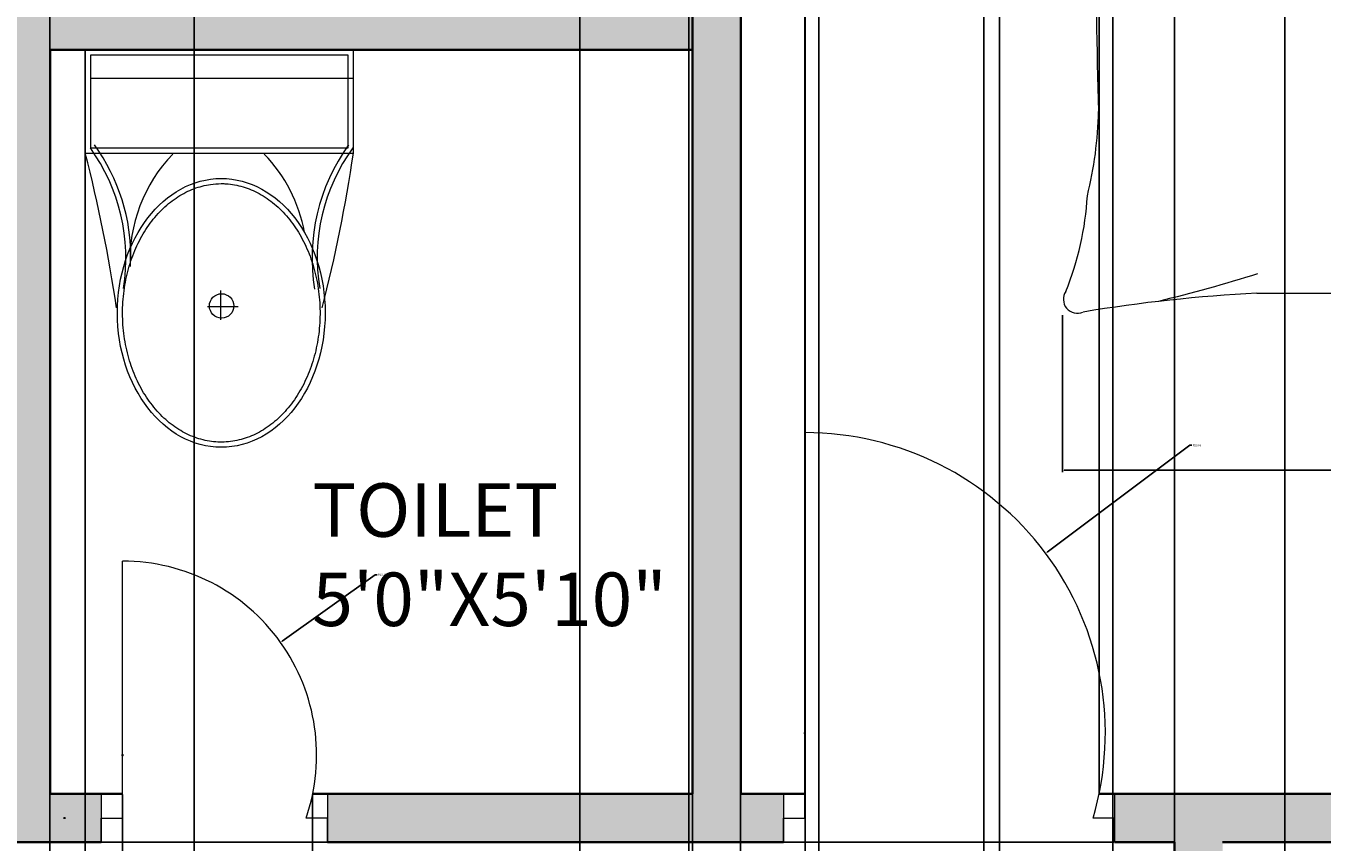
# Model space of a CAD drawing. Units: inches. Extents: x 2606 to 3027, y 1906 to 2463.
# Tile 7 of 10: x 2785 to 2906, y 2253 to 2329. Entities that reach past the tile are written whole.
import ezdxf

# ---------------------------------------------------------------- set-up
doc = ezdxf.new("R2010")
doc.units = ezdxf.units.IN
for name, color, linetype, lineweight in [('A-ANNO-DIMS', 2, 'Continuous', 18), ('A-AREA-IDEN', 7, 'Continuous', 18), ('A-DOOR', 3, 'Continuous', 18), ('A-FLOR-FIXT', 9, 'Continuous', 18), ('A-FURN', 8, 'Continuous', 13), ('A-WALL', 7, 'Continuous', 35)]:
    doc.layers.add(name, color=color, linetype=linetype, lineweight=lineweight)
doc.layers.add('A-WALL-PATT', color=251, linetype='Continuous', lineweight=13, true_color=0x636466)
doc.styles.get("Standard").update_dxf_attribs({"font": 'arial.ttf'})
doc.dimstyles.get("Standard").update_dxf_attribs({"dimtxt": 0.18, "dimasz": 0.18, "dimexe": 0.18, "dimexo": 0.0625, "dimgap": 0.09, "dimtad": 0, "dimtih": 1, "dimtoh": 1, "dimdec": 4, "dimzin": 0, "dimdsep": 46, "dimtxsty": 'Standard', "dimcen": 0.09, "dimadec": 0, "dimazin": 0, "dimtfac": 1, "dimtdec": 4, "dimtofl": 0, "dimtmove": 0, "dimatfit": 3, "dimfxl": 1, "dimtolj": 1, "dimtzin": 0, "dimarcsym": 0})

# ---------------------------------------------------------------- blocks, each defined once
blk = doc.blocks.new('A$C31115884')
for p, q in [((257.5, 466.4), (257.5, 523.2)), ((283.1, 497.7), (223.4, 497.7)), ((0, 200), (0, 0)), ((520, 200), (0, 200)), ((10, 190), (10, 10)), ((510, 190), (10, 190)), ((510, 10), (510, 190)), ((520, 0), (520, 200)), ((510, 54.5), (0, 54.5)), ((10, 10), (510, 10)), ((0, 0), (520, 0))]:
    blk.add_line(p, q)
blk.add_circle((255.6, 496.4), 23.6)
for centre, radius, start, end in [((2777.7, -204.6), 2807, 165.4549, 171.7133), ((3237, 905), 2807, 188.2867, 194.5451), ((-294.5, 403.3), 364.7, 324.2091, 9.3499), ((-294.5, 403.3), 374.7, 324.2091, 9.3499), ((805.8, 403.3), 364.7, 170.6501, 215.7909), ((139.5, 406.2), 293.5, 315.8436, 2.6563), ((805.8, 403.3), 374.7, 179.2036, 215.7909), ((383.6, 406.2), 293.5, 190.2774, 224.1564)]:
    blk.add_arc(centre, radius, start, end)
blk.add_ellipse((256.2, 509.9), major_axis=(0, -260.7), ratio=0.772727)
blk.add_open_spline([(256.2, 259.2), (263.1, 259.2), (270, 259.7), (287.8, 262.3), (298.7, 265.1), (319.9, 273.1), (330.2, 278.4), (350.1, 291.1), (359.7, 298.7), (377.7, 315.9), (386.2, 325.5), (401.7, 346.6), (408.8, 358.1), (421.3, 382.5), (426.8, 395.5), (435.9, 422.4), (439.5, 436.4), (444.8, 465.1), (446.5, 479.7), (447.9, 509.2), (447.6, 524), (445, 553.3), (442.7, 567.8), (436.3, 596), (432.1, 609.7), (421.9, 636), (416, 648.6), (402.5, 672.1), (395, 683), (378.6, 703), (369.8, 712.1), (351.1, 728), (341.3, 734.8), (320.9, 746.2), (310.4, 750.7), (288.9, 757.3), (278, 759.4), (256, 761), (245, 760.6), (223.1, 757.2), (212.3, 754.3), (191.1, 746.1), (180.8, 740.7), (160.9, 727.8), (151.4, 720.1), (133.5, 702.7), (125.1, 693), (109.6, 671.7), (102.6, 660.2), (90.2, 635.7), (84.9, 622.7), (76, 595.6), (72.4, 581.6), (67.2, 552.9), (65.6, 538.2), (64.4, 508.8), (64.8, 494), (67.5, 464.7), (69.9, 450.2), (76.6, 422), (80.8, 408.3), (91.1, 382.2), (97.2, 369.7), (110.8, 346.3), (118.4, 335.4), (134.8, 315.6), (143.7, 306.7), (162.4, 290.9), (172.3, 284.2), (192.8, 273), (203.3, 268.6), (224.8, 262.2), (235.8, 260.2), (249.9, 259.3), (253, 259.2), (256.2, 259.2)], degree=3, knots=[0, 0, 0, 0, 0.110105, 0.110105, 0.285049, 0.285049, 0.459994, 0.459994, 0.634938, 0.634938, 0.809882, 0.809882, 0.984827, 0.984827, 1.159771, 1.159771, 1.334715, 1.334715, 1.50966, 1.50966, 1.684604, 1.684604, 1.859549, 1.859549, 2.034493, 2.034493, 2.209437, 2.209437, 2.384382, 2.384382, 2.559326, 2.559326, 2.73427, 2.73427, 2.909215, 2.909215, 3.084159, 3.084159, 3.259103, 3.259103, 3.434048, 3.434048, 3.608992, 3.608992, 3.783936, 3.783936, 3.958881, 3.958881, 4.133825, 4.133825, 4.30877, 4.30877, 4.483714, 4.483714, 4.658658, 4.658658, 4.833603, 4.833603, 5.008547, 5.008547, 5.183491, 5.183491, 5.358436, 5.358436, 5.53338, 5.53338, 5.708324, 5.708324, 5.883269, 5.883269, 6.058213, 6.058213, 6.233158, 6.233158, 6.283185, 6.283185, 6.283185, 6.283185])
blk = doc.blocks.new('BED-DOUBLE')
for p, q in [((4.17, 75.16), (4.17, 96.87)), ((4.17, 96.87), (61.46, 96.87)), ((61.46, 96.87), (61.46, 64.97)), ((4.17, 95.03), (61.46, 95.03)), ((29.42, 93.94), (31.15, 94.63)), ((31.15, 94.63), (31.84, 88.22)), ((4.67, 92.87), (9.81, 93.27)), ((9.81, 93.27), (9.93, 93.24)), ((9.93, 93.24), (14.52, 92.9)), ((17.81, 92.38), (20.24, 93.24)), ((20.24, 93.24), (23.7, 94.11)), ((23.7, 94.11), (24.09, 94.11)), ((24.09, 94.11), (29.42, 93.94)), ((33.54, 93.89), (33.25, 87.44)), ((35.31, 93.3), (33.54, 93.89)), ((40.62, 93.81), (35.31, 93.3)), ((41.01, 93.83), (40.62, 93.81)), ((44.52, 93.18), (41.01, 93.83)), ((54.8, 93.82), (50.25, 93.19)), ((60.08, 93.81), (53.6, 93.92)), ((53.6, 93.92), (54.8, 93.82)), ((60.08, 93.81), (59.62, 89.96)), ((4.67, 92.9), (5.36, 89.08)), ((14.52, 92.9), (21.1, 91.68)), ((50.25, 93.19), (43.75, 91.57)), ((47, 92.47), (44.52, 93.18)), ((59.12, 86.97), (57.7, 90.18)), ((59.62, 89.96), (60.34, 86.88)), ((5.36, 89.08), (4.84, 85.96)), ((6.06, 86.14), (7.27, 89.43)), ((31.84, 88.22), (32.54, 84.4)), ((33.25, 87.44), (32.79, 83.59)), ((4.84, 85.96), (5.54, 84.75)), ((5.36, 81.8), (6.06, 86.14)), ((60.08, 82.69), (59.12, 86.97)), ((60.34, 86.88), (59.72, 85.62)), ((32.54, 84.4), (32.54, 82.84)), ((32.79, 83.59), (32.89, 82.03)), ((32.54, 82.84), (31.84, 80.59)), ((59.85, 80.77), (60.08, 82.69)), ((5.71, 79.9), (5.36, 81.8)), ((32.89, 82.03), (33.72, 79.83)), ((5.02, 76.08), (5.71, 79.9)), ((31.84, 80.59), (31.84, 77.38)), ((60.78, 77), (59.85, 80.77)), ((28.9, 77.38), (25.13, 78.68)), ((33.72, 79.83), (33.92, 76.62)), ((7.65, 78.14), (12.48, 77.34)), ((20.89, 76.82), (23.24, 77.49)), ((23.24, 77.49), (29.39, 77)), ((36.87, 76.8), (40.55, 78.34)), ((39.04, 78.14), (43.87, 77.34)), ((52.28, 76.82), (54.63, 77.49)), ((54.63, 77.49), (60.78, 77)), ((11.13, 76.95), (5.02, 76.08)), ((12.48, 77.34), (11.13, 76.95)), ((12.48, 77.34), (20.89, 76.82)), ((31.84, 77.38), (28.9, 77.38)), ((33.92, 76.62), (36.87, 76.8)), ((43.87, 77.34), (52.28, 76.82)), ((36.28, 76.03), (41.3, 68.25)), ((48.73, 72.52), (38.73, 76.03)), ((55.41, 70.1), (48.73, 72.52)), ((58.94, 67.51), (55.41, 70.1)), ((41.3, 68.25), (43.34, 62.87)), ((63.38, 63.61), (58.94, 67.51)), ((53.18, 62.87), (57.82, 63.24)), ((57.82, 63.24), (61.54, 62.87)), ((61.54, 62.87), (63.38, 63.61)), ((63.48, 61.52), (63.38, 63.61, 4.64)), ((43.34, 62.87), (43.71, 60.45)), ((46.68, 61.2), (49.1, 62.31)), ((49.1, 62.31), (53.18, 62.87)), ((43.71, 60.45), (46.68, 61.2)), ((18.06, 1.87), (47.57, 1.87))]:
    blk.add_line(p, q)
for centre, radius, start, end in [((25.61, -121.38), 197.77, 86.0865, 96.7821), ((102.1, 72.78), 99.87, 178.7218, 185.604), ((21.29, -90.53), 154.68, 81.7845, 96.9006), ((-200.58, 59.5), 203.94, 358.4762, 1.0082), ((52.44, 54.83), 7.46, 78.6608, 113.7384), ((61.53, 104.85), 43.38, 259.8763, 272.5657), ((37.35, 95.1), 35.55, 280.6617, 289.8806), ((218.51, 53.34), 155.25, 176.9791, 183.8365), ((43.92, 60.38), 0.221, 160.2464, 271.1377), ((581.23, 36.19), 578.22, 178.22771, 181.71854), ((-5405.34, 15.56), 5469.02, 0.00217, 0.28689), ((-32.25, 19.53), 35.53, 346.0648, 358.9113), ((91.3, 14.55), 27.65, 177.4714, 206.4681), ((-25.97, 12.62), 28.25, 337.9751, 356.652), ((-20.65, 125.3), 127.63, 283.3832, 287.7053), ((1.3, 1.3), 1.31, 146.1736, 293.4781), ((25.69, -143.9), 145.97, 92.9958, 99.4091), ((49.34, -157.62), 159.5, 84.4998, 90.6351), ((65.23, 2.32), 1.32, 242.6588, 356.02)]:
    blk.add_arc(centre, radius, start, end)
blk = doc.blocks.new('*D10')
at = {"layer": 'A-ANNO-DIMS', "color": 0, "lineweight": -2, "transparency": 16777216}
for p, q in [((2882.1, 2302.34), (2882.1, 2287.67)), ((2948.75, 2302.34), (2948.75, 2287.67)), ((2882.28, 2287.85), (2914.9, 2287.85)), ((2948.57, 2287.85), (2915.96, 2287.85))]:
    blk.add_line(p, q, dxfattribs=at)
at = {"layer": 'A-ANNO-DIMS', "color": 0, "transparency": 16777216}
for points in [[(2882.28, 2287.88), (2882.28, 2287.82), (2882.1, 2287.85)], [(2948.57, 2287.88), (2948.57, 2287.82), (2948.75, 2287.85)]]:
    blk.add_solid(points, dxfattribs=at)
at = {"layer": 'Defpoints', "color": 0, "transparency": 16777216}
for p in [(2882.1, 2302.4), (2948.75, 2302.4), (2948.75, 2287.85)]:
    blk.add_point(p, dxfattribs=at)
at = {"layer": 'A-ANNO-DIMS', "color": 0, "transparency": 16777216, "insert": (2915.43, 2287.85), "char_height": 0.18, "attachment_point": 5}
blk.add_mtext('\\A1;67 TYP.', dxfattribs=at)
blk = doc.blocks.new('*D34')
at = {"layer": 'A-ANNO-DIMS', "color": 0, "lineweight": -2, "transparency": 16777216}
for p, q in [((2787.56, 2118.27), (2787.56, 2433.99)), ((2787.74, 2433.81), (2817.34, 2433.81)), ((2847.38, 2433.81), (2817.78, 2433.81)), ((2847.56, 2118.27), (2847.56, 2433.99))]:
    blk.add_line(p, q, dxfattribs=at)
at = {"layer": 'A-ANNO-DIMS', "color": 0, "transparency": 16777216}
for points in [[(2787.74, 2433.84), (2787.74, 2433.78), (2787.56, 2433.81)], [(2847.38, 2433.84), (2847.38, 2433.78), (2847.56, 2433.81)]]:
    blk.add_solid(points, dxfattribs=at)
at = {"layer": 'Defpoints', "color": 0, "transparency": 16777216}
for p in [(2847.56, 2433.81), (2787.56, 2118.21), (2847.56, 2118.21)]:
    blk.add_point(p, dxfattribs=at)
at = {"layer": 'A-ANNO-DIMS', "color": 0, "transparency": 16777216, "insert": (2817.56, 2433.81), "char_height": 0.18, "attachment_point": 5}
blk.add_mtext('\\A1;60', dxfattribs=at)
blk = doc.blocks.new('*D35')
at = {"layer": 'A-ANNO-DIMS', "color": 0, "lineweight": -2, "transparency": 16777216}
for p, q in [((2801.04, 1993.17), (2801.04, 2433.99)), ((2801.22, 2433.81), (2818.82, 2433.81)), ((2836.86, 2433.81), (2819.26, 2433.81)), ((2837.04, 1993.17), (2837.04, 2433.99))]:
    blk.add_line(p, q, dxfattribs=at)
at = {"layer": 'A-ANNO-DIMS', "color": 0, "transparency": 16777216}
for points in [[(2801.22, 2433.84), (2801.22, 2433.78), (2801.04, 2433.81)], [(2836.86, 2433.84), (2836.86, 2433.78), (2837.04, 2433.81)]]:
    blk.add_solid(points, dxfattribs=at)
at = {"layer": 'Defpoints', "color": 0, "transparency": 16777216}
for p in [(2837.04, 2433.81), (2801.04, 1993.11), (2837.04, 1993.11)]:
    blk.add_point(p, dxfattribs=at)
at = {"layer": 'A-ANNO-DIMS', "color": 0, "transparency": 16777216, "insert": (2819.04, 2433.81), "char_height": 0.18, "attachment_point": 5}
blk.add_mtext('\\A1;36', dxfattribs=at)
blk = doc.blocks.new('*D36')
at = {"layer": 'A-ANNO-DIMS', "color": 0, "lineweight": -2, "transparency": 16777216}
for p, q in [((2787.56, 1993.17), (2787.56, 2433.99)), ((2787.74, 2433.81), (2793.85, 2433.81)), ((2800.86, 2433.81), (2794.76, 2433.81)), ((2801.04, 1993.17), (2801.04, 2433.99))]:
    blk.add_line(p, q, dxfattribs=at)
at = {"layer": 'A-ANNO-DIMS', "color": 0, "transparency": 16777216}
for points in [[(2787.74, 2433.84), (2787.74, 2433.78), (2787.56, 2433.81)], [(2800.86, 2433.84), (2800.86, 2433.78), (2801.04, 2433.81)]]:
    blk.add_solid(points, dxfattribs=at)
at = {"layer": 'Defpoints', "color": 0, "transparency": 16777216}
for p in [(2787.56, 2433.81), (2787.56, 1993.11), (2801.04, 1993.11)]:
    blk.add_point(p, dxfattribs=at)
at = {"layer": 'A-ANNO-DIMS', "color": 0, "transparency": 16777216, "insert": (2794.3, 2433.81), "char_height": 0.18, "attachment_point": 5}
blk.add_mtext('\\A1;13.478', dxfattribs=at)
blk = doc.blocks.new('*D38')
at = {"layer": 'A-ANNO-DIMS', "color": 0, "lineweight": -2, "transparency": 16777216}
for p, q in [((2783.06, 1993.17), (2783.06, 2433.99)), ((2783.24, 2433.81), (2785.05, 2433.81)), ((2787.38, 2433.81), (2785.57, 2433.81)), ((2787.56, 1993.17), (2787.56, 2433.99))]:
    blk.add_line(p, q, dxfattribs=at)
at = {"layer": 'A-ANNO-DIMS', "color": 0, "transparency": 16777216}
for points in [[(2783.24, 2433.84), (2783.24, 2433.78), (2783.06, 2433.81)], [(2787.38, 2433.84), (2787.38, 2433.78), (2787.56, 2433.81)]]:
    blk.add_solid(points, dxfattribs=at)
at = {"layer": 'Defpoints', "color": 0, "transparency": 16777216}
for p in [(2787.56, 2433.81), (2783.06, 1993.11), (2787.56, 1993.11)]:
    blk.add_point(p, dxfattribs=at)
at = {"layer": 'A-ANNO-DIMS', "color": 0, "transparency": 16777216, "insert": (2785.31, 2433.81), "char_height": 0.18, "attachment_point": 5}
blk.add_mtext('\\A1;4.5', dxfattribs=at)
blk = doc.blocks.new('*D43')
at = {"layer": 'A-ANNO-DIMS', "color": 0, "lineweight": -2, "transparency": 16777216}
for p, q in [((2794.34, 2257.55), (2794.34, 1965.23)), ((2812.09, 2257.55), (2812.09, 1965.23)), ((2794.52, 1965.41), (2802.76, 1965.41)), ((2811.91, 1965.41), (2803.67, 1965.41))]:
    blk.add_line(p, q, dxfattribs=at)
at = {"layer": 'A-ANNO-DIMS', "color": 0, "transparency": 16777216}
for points in [[(2794.52, 1965.44), (2794.52, 1965.38), (2794.34, 1965.41)], [(2811.91, 1965.44), (2811.91, 1965.38), (2812.09, 1965.41)]]:
    blk.add_solid(points, dxfattribs=at)
at = {"layer": 'Defpoints', "color": 0, "transparency": 16777216}
for p in [(2794.34, 2257.61), (2812.09, 2257.61), (2812.09, 1965.41)]:
    blk.add_point(p, dxfattribs=at)
at = {"layer": 'A-ANNO-DIMS', "color": 0, "transparency": 16777216, "insert": (2803.22, 1965.41), "char_height": 0.18, "attachment_point": 5}
blk.add_mtext('\\A1;17.756', dxfattribs=at)
blk = doc.blocks.new('*D44')
at = {"layer": 'A-ANNO-DIMS', "color": 0, "lineweight": -2, "transparency": 16777216}
for p, q in [((2858.06, 2257.67), (2858.06, 2433.99)), ((2858.24, 2433.81), (2871.33, 2433.81)), ((2885.35, 2433.81), (2872.26, 2433.81)), ((2885.53, 2257.67), (2885.53, 2433.99))]:
    blk.add_line(p, q, dxfattribs=at)
at = {"layer": 'A-ANNO-DIMS', "color": 0, "transparency": 16777216}
for points in [[(2858.24, 2433.84), (2858.24, 2433.78), (2858.06, 2433.81)], [(2885.35, 2433.84), (2885.35, 2433.78), (2885.53, 2433.81)]]:
    blk.add_solid(points, dxfattribs=at)
at = {"layer": 'Defpoints', "color": 0, "transparency": 16777216}
for p in [(2885.53, 2433.81), (2858.06, 2257.61), (2885.53, 2257.61)]:
    blk.add_point(p, dxfattribs=at)
at = {"layer": 'A-ANNO-DIMS', "color": 0, "transparency": 16777216, "insert": (2871.79, 2433.81), "char_height": 0.18, "attachment_point": 5}
blk.add_mtext('\\A1;27.475', dxfattribs=at)
blk = doc.blocks.new('*D46')
at = {"layer": 'A-ANNO-DIMS', "color": 0, "lineweight": -2, "transparency": 16777216}
for p, q in [((2859.37, 2154.92), (2859.37, 2433.99)), ((2859.55, 2433.81), (2872.63, 2433.81)), ((2886.63, 2433.81), (2873.56, 2433.81)), ((2886.81, 2157.17), (2886.81, 2433.99))]:
    blk.add_line(p, q, dxfattribs=at)
at = {"layer": 'A-ANNO-DIMS', "color": 0, "transparency": 16777216}
for points in [[(2859.55, 2433.84), (2859.55, 2433.78), (2859.37, 2433.81)], [(2886.63, 2433.84), (2886.63, 2433.78), (2886.81, 2433.81)]]:
    blk.add_solid(points, dxfattribs=at)
at = {"layer": 'Defpoints', "color": 0, "transparency": 16777216}
for p in [(2886.81, 2433.81), (2886.81, 2157.11), (2859.37, 2154.86)]:
    blk.add_point(p, dxfattribs=at)
at = {"layer": 'A-ANNO-DIMS', "color": 0, "transparency": 16777216, "insert": (2873.09, 2433.81), "char_height": 0.18, "attachment_point": 5}
blk.add_mtext('\\A1;27.443', dxfattribs=at)
blk = doc.blocks.new('*D48')
at = {"layer": 'A-ANNO-DIMS', "color": 0, "lineweight": -2, "transparency": 16777216}
for p, q in [((2858.07, 2028.17), (2858.07, 2433.99)), ((2858.25, 2433.81), (2866.77, 2433.81)), ((2876.06, 2433.81), (2867.54, 2433.81)), ((2876.24, 2028.17), (2876.24, 2433.99))]:
    blk.add_line(p, q, dxfattribs=at)
at = {"layer": 'A-ANNO-DIMS', "color": 0, "transparency": 16777216}
for points in [[(2858.25, 2433.84), (2858.25, 2433.78), (2858.07, 2433.81)], [(2876.06, 2433.84), (2876.06, 2433.78), (2876.24, 2433.81)]]:
    blk.add_solid(points, dxfattribs=at)
at = {"layer": 'Defpoints', "color": 0, "transparency": 16777216}
for p in [(2876.24, 2433.81), (2858.07, 2028.11), (2876.24, 2028.11)]:
    blk.add_point(p, dxfattribs=at)
at = {"layer": 'A-ANNO-DIMS', "color": 0, "transparency": 16777216, "insert": (2867.16, 2433.81), "char_height": 0.18, "attachment_point": 5}
blk.add_mtext('\\A1;18.17', dxfattribs=at)
blk = doc.blocks.new('*D51')
at = {"layer": 'A-ANNO-DIMS', "color": 0, "lineweight": -2, "transparency": 16777216}
for p, q in [((2852.06, 2257.67), (2852.06, 2433.99)), ((2852.24, 2433.81), (2854.67, 2433.81)), ((2857.88, 2433.81), (2855.45, 2433.81)), ((2858.06, 2257.67), (2858.06, 2433.99))]:
    blk.add_line(p, q, dxfattribs=at)
at = {"layer": 'A-ANNO-DIMS', "color": 0, "transparency": 16777216}
for points in [[(2852.24, 2433.84), (2852.24, 2433.78), (2852.06, 2433.81)], [(2857.88, 2433.84), (2857.88, 2433.78), (2858.06, 2433.81)]]:
    blk.add_solid(points, dxfattribs=at)
at = {"layer": 'Defpoints', "color": 0, "transparency": 16777216}
for p in [(2858.06, 2433.81), (2852.06, 2257.61), (2858.06, 2257.61)]:
    blk.add_point(p, dxfattribs=at)
at = {"layer": 'A-ANNO-DIMS', "color": 0, "transparency": 16777216, "insert": (2855.06, 2433.81), "char_height": 0.18, "attachment_point": 5}
blk.add_mtext('\\A1;5.994', dxfattribs=at)
blk = doc.blocks.new('*D52')
at = {"layer": 'A-ANNO-DIMS', "color": 0, "lineweight": -2, "transparency": 16777216}
for p, q in [((2787.56, 2257.55), (2787.56, 1965.23)), ((2794.34, 2257.55), (2794.34, 1965.23)), ((2787.74, 1965.41), (2790.56, 1965.41)), ((2794.16, 1965.41), (2791.34, 1965.41))]:
    blk.add_line(p, q, dxfattribs=at)
at = {"layer": 'A-ANNO-DIMS', "color": 0, "transparency": 16777216}
for points in [[(2787.74, 1965.44), (2787.74, 1965.38), (2787.56, 1965.41)], [(2794.16, 1965.44), (2794.16, 1965.38), (2794.34, 1965.41)]]:
    blk.add_solid(points, dxfattribs=at)
at = {"layer": 'Defpoints', "color": 0, "transparency": 16777216}
for p in [(2787.56, 2257.61), (2794.34, 2257.61), (2794.34, 1965.41)]:
    blk.add_point(p, dxfattribs=at)
at = {"layer": 'A-ANNO-DIMS', "color": 0, "transparency": 16777216, "insert": (2790.95, 1965.41), "char_height": 0.18, "attachment_point": 5}
blk.add_mtext('\\A1;6.776', dxfattribs=at)
blk = doc.blocks.new('*D55')
at = {"layer": 'A-ANNO-DIMS', "color": 0, "lineweight": -2, "transparency": 16777216}
for p, q in [((2852.06, 2152.67), (2852.06, 2433.99)), ((2852.24, 2433.81), (2855.32, 2433.81)), ((2859.19, 2433.81), (2856.11, 2433.81)), ((2859.37, 2154.92), (2859.37, 2433.99))]:
    blk.add_line(p, q, dxfattribs=at)
at = {"layer": 'A-ANNO-DIMS', "color": 0, "transparency": 16777216}
for points in [[(2852.24, 2433.84), (2852.24, 2433.78), (2852.06, 2433.81)], [(2859.19, 2433.84), (2859.19, 2433.78), (2859.37, 2433.81)]]:
    blk.add_solid(points, dxfattribs=at)
at = {"layer": 'Defpoints', "color": 0, "transparency": 16777216}
for p in [(2859.37, 2433.81), (2859.37, 2154.86), (2852.06, 2152.61)]:
    blk.add_point(p, dxfattribs=at)
at = {"layer": 'A-ANNO-DIMS', "color": 0, "transparency": 16777216, "insert": (2855.72, 2433.81), "char_height": 0.18, "attachment_point": 5}
blk.add_mtext('\\A1;7.306', dxfattribs=at)
blk = doc.blocks.new('*D57')
at = {"layer": 'A-ANNO-DIMS', "color": 0, "lineweight": -2, "transparency": 16777216}
for p, q in [((2876.24, 2028.17), (2876.24, 2433.99)), ((2876.42, 2433.81), (2889.17, 2433.81)), ((2902.71, 2433.81), (2889.96, 2433.81)), ((2902.89, 2028.17), (2902.89, 2433.99))]:
    blk.add_line(p, q, dxfattribs=at)
at = {"layer": 'A-ANNO-DIMS', "color": 0, "transparency": 16777216}
for points in [[(2876.42, 2433.84), (2876.42, 2433.78), (2876.24, 2433.81)], [(2902.71, 2433.84), (2902.71, 2433.78), (2902.89, 2433.81)]]:
    blk.add_solid(points, dxfattribs=at)
at = {"layer": 'Defpoints', "color": 0, "transparency": 16777216}
for p in [(2902.89, 2433.81), (2876.24, 2028.11), (2902.89, 2028.11)]:
    blk.add_point(p, dxfattribs=at)
at = {"layer": 'A-ANNO-DIMS', "color": 0, "transparency": 16777216, "insert": (2889.57, 2433.81), "char_height": 0.18, "attachment_point": 5}
blk.add_mtext('\\A1;26.65', dxfattribs=at)
blk = doc.blocks.new('*D70')
at = {"layer": 'A-ANNO-DIMS', "color": 0, "lineweight": -2, "transparency": 16777216}
for p, q in [((2847.23, 2221.7), (2847.23, 2433.99)), ((2847.41, 2433.81), (2860.54, 2433.81)), ((2874.6, 2433.81), (2861.47, 2433.81)), ((2874.78, 2221.7), (2874.78, 2433.99))]:
    blk.add_line(p, q, dxfattribs=at)
at = {"layer": 'A-ANNO-DIMS', "color": 0, "transparency": 16777216}
for points in [[(2847.41, 2433.84), (2847.41, 2433.78), (2847.23, 2433.81)], [(2874.6, 2433.84), (2874.6, 2433.78), (2874.78, 2433.81)]]:
    blk.add_solid(points, dxfattribs=at)
at = {"layer": 'Defpoints', "color": 0, "transparency": 16777216}
for p in [(2874.78, 2433.81), (2847.23, 2221.64), (2874.78, 2221.64)]:
    blk.add_point(p, dxfattribs=at)
at = {"layer": 'A-ANNO-DIMS', "color": 0, "transparency": 16777216, "insert": (2861, 2433.81), "char_height": 0.18, "attachment_point": 5}
blk.add_mtext('\\A1;27.555', dxfattribs=at)
blk = doc.blocks.new('*D72')
at = {"layer": 'A-ANNO-DIMS', "color": 0, "lineweight": -2, "transparency": 16777216}
for p, q in [((2874.78, 2221.7), (2874.78, 2433.99)), ((2874.96, 2433.81), (2883.22, 2433.81)), ((2892.38, 2433.81), (2884.13, 2433.81)), ((2892.56, 2215.2), (2892.56, 2433.99))]:
    blk.add_line(p, q, dxfattribs=at)
at = {"layer": 'A-ANNO-DIMS', "color": 0, "transparency": 16777216}
for points in [[(2874.96, 2433.84), (2874.96, 2433.78), (2874.78, 2433.81)], [(2892.38, 2433.84), (2892.38, 2433.78), (2892.56, 2433.81)]]:
    blk.add_solid(points, dxfattribs=at)
at = {"layer": 'Defpoints', "color": 0, "transparency": 16777216}
for p in [(2892.56, 2433.81), (2874.78, 2221.64), (2892.56, 2215.13)]:
    blk.add_point(p, dxfattribs=at)
at = {"layer": 'A-ANNO-DIMS', "color": 0, "transparency": 16777216, "insert": (2883.67, 2433.81), "char_height": 0.18, "attachment_point": 5}
blk.add_mtext('\\A1;17.783', dxfattribs=at)
blk = doc.blocks.new('*D73')
at = {"layer": 'A-ANNO-DIMS', "color": 0, "lineweight": -2, "transparency": 16777216}
for p, q in [((2886.91, 2253.11), (2634.68, 2253.11)), ((2634.86, 2252.93), (2634.86, 2237.56)), ((2634.86, 2221.82), (2634.86, 2237.19)), ((2847.16, 2221.64), (2634.68, 2221.64))]:
    blk.add_line(p, q, dxfattribs=at)
at = {"layer": 'A-ANNO-DIMS', "color": 0, "transparency": 16777216}
for points in [[(2634.83, 2252.93), (2634.89, 2252.93), (2634.86, 2253.11)], [(2634.83, 2221.82), (2634.89, 2221.82), (2634.86, 2221.64)]]:
    blk.add_solid(points, dxfattribs=at)
at = {"layer": 'Defpoints', "color": 0, "transparency": 16777216}
for p in [(2634.86, 2253.11), (2886.97, 2253.11), (2847.23, 2221.64)]:
    blk.add_point(p, dxfattribs=at)
at = {"layer": 'A-ANNO-DIMS', "color": 0, "transparency": 16777216, "insert": (2634.86, 2237.37), "char_height": 0.18, "attachment_point": 5}
blk.add_mtext('\\A1;31.47', dxfattribs=at)
blk = doc.blocks.new('*D83')
at = {"layer": 'A-ANNO-DIMS', "color": 0, "lineweight": -2, "transparency": 16777216}
for p, q in [((2787.56, 2327.05), (2787.56, 1965.23)), ((2790.85, 2327.05), (2790.85, 1965.23)), ((2787.74, 1965.41), (2788.88, 1965.41)), ((2790.67, 1965.41), (2789.53, 1965.41))]:
    blk.add_line(p, q, dxfattribs=at)
at = {"layer": 'A-ANNO-DIMS', "color": 0, "transparency": 16777216}
for points in [[(2787.74, 1965.44), (2787.74, 1965.38), (2787.56, 1965.41)], [(2790.67, 1965.44), (2790.67, 1965.38), (2790.85, 1965.41)]]:
    blk.add_solid(points, dxfattribs=at)
at = {"layer": 'Defpoints', "color": 0, "transparency": 16777216}
for p in [(2787.56, 2327.11), (2790.85, 2327.11), (2790.85, 1965.41)]:
    blk.add_point(p, dxfattribs=at)
at = {"layer": 'A-ANNO-DIMS', "color": 0, "transparency": 16777216, "insert": (2789.21, 1965.41), "char_height": 0.18, "attachment_point": 5}
blk.add_mtext('\\A1;3.29', dxfattribs=at)
blk = doc.blocks.new('*D84')
at = {"layer": 'A-ANNO-DIMS', "color": 0, "lineweight": -2, "transparency": 16777216}
for p, q in [((2739.27, 2290.79), (2739.45, 2290.79)), ((2739.45, 2290.79), (2757.85, 2277.61)), ((2788.82, 2255.36), (2789, 2255.36)), ((2788.91, 2255.27), (2788.91, 2255.45))]:
    blk.add_line(p, q, dxfattribs=at)
at = {"layer": 'A-ANNO-DIMS', "color": 0, "transparency": 16777216}
blk.add_solid([(2757.87, 2277.63), (2757.84, 2277.58), (2758, 2277.5)], dxfattribs=at)
at = {"layer": 'Defpoints', "color": 0, "transparency": 16777216}
for p in [(2758, 2277.5), (2788.91, 2255.36)]:
    blk.add_point(p, dxfattribs=at)
at = {"layer": 'A-ANNO-DIMS', "color": 0, "transparency": 16777216, "insert": (2738.79, 2290.79), "char_height": 0.18, "attachment_point": 5}
blk.add_mtext('\\A1;R38.02', dxfattribs=at)
blk = doc.blocks.new('*D85')
at = {"layer": 'A-ANNO-DIMS', "color": 0, "lineweight": -2, "transparency": 16777216}
for p, q in [((2894.01, 2290.18), (2880.67, 2280.21)), ((2894.19, 2290.18), (2894.01, 2290.18)), ((2857.97, 2263.3), (2858.15, 2263.3)), ((2858.06, 2263.21), (2858.06, 2263.39))]:
    blk.add_line(p, q, dxfattribs=at)
at = {"layer": 'A-ANNO-DIMS', "color": 0, "transparency": 16777216}
blk.add_solid([(2880.66, 2280.23), (2880.69, 2280.18), (2880.53, 2280.1)], dxfattribs=at)
at = {"layer": 'Defpoints', "color": 0, "transparency": 16777216}
for p in [(2880.53, 2280.1), (2858.06, 2263.3)]:
    blk.add_point(p, dxfattribs=at)
at = {"layer": 'A-ANNO-DIMS', "color": 0, "transparency": 16777216, "insert": (2894.67, 2290.18), "char_height": 0.18, "attachment_point": 5}
blk.add_mtext('\\A1;R28.06', dxfattribs=at)
blk = doc.blocks.new('*D91')
at = {"layer": 'A-ANNO-DIMS', "color": 0, "lineweight": -2, "transparency": 16777216}
for p, q in [((2817.93, 2278.09), (2809.23, 2271.88)), ((2818.11, 2278.09), (2817.93, 2278.09)), ((2794.25, 2261.24), (2794.43, 2261.24)), ((2794.34, 2261.15), (2794.34, 2261.33))]:
    blk.add_line(p, q, dxfattribs=at)
at = {"layer": 'A-ANNO-DIMS', "color": 0, "transparency": 16777216}
blk.add_solid([(2809.21, 2271.9), (2809.25, 2271.85), (2809.09, 2271.77)], dxfattribs=at)
at = {"layer": 'Defpoints', "color": 0, "transparency": 16777216}
for p in [(2809.09, 2271.77), (2794.34, 2261.24)]:
    blk.add_point(p, dxfattribs=at)
at = {"layer": 'A-ANNO-DIMS', "color": 0, "transparency": 16777216, "insert": (2818.66, 2278.09), "char_height": 0.18, "attachment_point": 5}
blk.add_mtext('\\A1;R18.123', dxfattribs=at)

msp = doc.modelspace()

# ---------------------------------------------------------------- hatches: boundary and pattern name
at = {"layer": 'A-WALL-PATT'}
h = msp.add_hatch(color=256, dxfattribs=at)
h.dxf.hatch_style = 1
h.paths.add_polyline_path([(2667.063, 2401.6097), (2691.9697, 2401.6097), (2691.9697, 2406.1097), (2691.9697, 2410.6097), (2658.063, 2410.6097), (2658.063, 2238.7051), (2667.063, 2238.7051)])
h.paths.add_polyline_path([(2804.9965, 2406.1097), (2804.9965, 2410.6097), (2751.9697, 2410.6097), (2751.9697, 2401.6097), (2783.063, 2401.6097), (2783.063, 2257.6097), (2778.6739, 2257.6097), (2778.6739, 2253.1097), (2792.3386, 2253.1097), (2792.3386, 2255.3597), (2792.3386, 2257.6097), (2787.563, 2257.6097), (2787.563, 2327.1097), (2847.563, 2327.1097), (2847.563, 2331.6097), (2787.563, 2331.6097), (2787.563, 2401.6097), (2804.9965, 2401.6097)])
h.paths.add_polyline_path([(2889.6183, 2406.1097), (2889.6183, 2410.6097), (2828.9965, 2410.6097), (2828.9965, 2401.6097), (2831.8174, 2401.6097), (2847.563, 2401.6097), (2847.563, 2357.8311), (2849.813, 2357.8311), (2852.063, 2357.8311), (2852.063, 2401.6097), (2889.6183, 2401.6097)])
h.paths.add_polyline_path([(2977.063, 2410.6097), (2949.6183, 2410.6097), (2949.6183, 2401.6097), (2968.063, 2401.6097), (2968.063, 2157.1097), (2897.063, 2157.1097), (2897.063, 2174.1966), (2892.563, 2174.1966), (2892.563, 2157.1097), (2886.8122, 2157.1097), (2886.8122, 2152.6097), (2968.063, 2152.6097), (2968.063, 2032.6097), (2950.8911, 2032.6097), (2950.8911, 2028.1097), (2968.063, 2028.1097), (2968.063, 1993.1097), (2852.063, 1993.1097), (2852.063, 2028.1097), (2856.0743, 2028.1097), (2856.0743, 2030.3597), (2856.0743, 2032.6097), (2852.063, 2032.6097), (2852.063, 2152.6097), (2857.369, 2152.6097), (2857.369, 2154.8597), (2857.369, 2157.1097), (2847.563, 2157.1097), (2847.563, 2152.6097), (2847.563, 1993.1097), (2837.0415, 1993.1097), (2837.0415, 1988.6097), (2977.063, 1988.6097)])
h.paths.add_polyline_path([(2968.063, 2257.6097), (2886.9679, 2257.6097), (2886.9679, 2253.1097), (2892.563, 2253.1097), (2892.563, 2215.1332), (2897.063, 2215.1332), (2897.063, 2253.1097), (2968.063, 2253.1097)], flags=17)
h.paths.add_polyline_path([(2856.057, 2255.3597), (2856.057, 2257.6097), (2852.063, 2257.6097), (2852.063, 2336.7476), (2849.813, 2336.7476), (2847.563, 2336.7476), (2847.563, 2331.6097), (2847.563, 2327.1097), (2847.563, 2257.6097), (2813.482, 2257.6097), (2813.482, 2253.1097), (2856.057, 2253.1097)])
h.paths.add_polyline_path([(2748.8874, 2255.3597), (2748.8874, 2257.6097), (2667.063, 2257.6097), (2667.063, 2253.1097), (2748.8874, 2253.1097)])
h.paths.add_polyline_path([(2667.063, 2152.6097), (2744.8238, 2152.6097), (2744.8238, 2154.8597), (2744.8238, 2157.1097), (2667.063, 2157.1097), (2667.063, 2178.7051), (2658.063, 2178.7051), (2658.063, 1988.6097), (2801.0415, 1988.6097), (2801.0415, 1990.8597), (2801.0415, 1993.1097), (2787.563, 1993.1097), (2787.563, 2157.1097), (2777.1295, 2157.1097), (2777.1295, 2152.6097), (2783.063, 2152.6097), (2783.063, 2032.6097), (2778.4484, 2032.6097), (2778.4484, 2028.1097), (2783.063, 2028.1097), (2783.063, 1993.1097), (2667.063, 1993.1097), (2667.063, 2028.1097), (2680.1652, 2028.1097), (2680.1652, 2030.3597), (2680.1652, 2032.6097), (2667.063, 2032.6097)])
h.paths.add_polyline_path([(2755.4074, 2032.6097), (2728.1652, 2032.6097), (2728.1652, 2028.1097), (2755.4074, 2028.1097), (2755.4074, 2030.3597)], flags=17)
h.paths.add_polyline_path([(2902.8911, 2030.3597), (2902.8911, 2032.6097), (2877.6885, 2032.6097), (2877.6885, 2028.1097), (2902.8911, 2028.1097)], flags=17)
h.paths.add_polyline_path([(2810.2211, 2267.221), (2851.2716, 2267.221), (2851.2716, 2289.6098), (2810.2211, 2289.6098)], flags=9)
h = msp.add_hatch(color=256, dxfattribs=at)
h.dxf.hatch_style = 1
h.paths.add_polyline_path([(2852.063, 2336.7476), (2849.813, 2336.7476), (2847.563, 2336.7476), (2847.563, 2331.6097), (2847.563, 2257.6097), (2813.482, 2257.6097), (2813.482, 2253.1097), (2856.057, 2253.1097), (2856.057, 2255.3597), (2856.057, 2257.6097), (2852.063, 2257.6097)])

# ---------------------------------------------------------------- linework, layer by layer
at = {"layer": 'A-DOOR'}
for p, q in [((2858.057, 2255.3597), (2858.057, 2291.3597)), ((2794.3386, 2255.3597), (2794.3386, 2279.3597)), ((2792.3386, 2257.6097), (2792.3386, 2253.1097)), ((2813.482, 2257.6097), (2813.482, 2253.1097)), ((2856.057, 2257.6097), (2856.057, 2253.1097)), ((2886.9679, 2257.6097), (2886.9679, 2253.1097)), ((2792.3386, 2253.1097), (2792.3386, 2255.3597)), ((2792.3386, 2255.3597), (2794.3386, 2255.3597)), ((2813.482, 2255.3597), (2811.482, 2255.3597)), ((2813.482, 2253.1097), (2813.482, 2255.3597)), ((2856.057, 2253.1097), (2856.057, 2255.3597)), ((2856.057, 2255.3597), (2858.057, 2255.3597)), ((2886.9679, 2255.3597), (2884.9679, 2255.3597)), ((2886.9679, 2253.1097), (2886.9679, 2255.3597))]:
    msp.add_line(p, q, dxfattribs=at)
for centre, radius, start in [((2858.057, 2263.3014), 28.0582, 343.557963), ((2794.3386, 2261.2369), 18.1228, 341.076976)]:
    msp.add_arc(centre, radius, start, 90, dxfattribs=at)
at = {"layer": 'A-WALL'}
for p, q in [((2847.563, 2338.7476), (2847.563, 2257.6097)), ((2852.063, 2336.7476), (2852.063, 2257.6097)), ((2787.563, 2327.1097), (2847.563, 2327.1097)), ((2787.563, 2327.1097), (2787.563, 2257.6097)), ((2787.563, 2257.6097), (2794.3386, 2257.6097)), ((2812.0947, 2257.6097), (2847.563, 2257.6097)), ((2852.063, 2257.6097), (2858.057, 2257.6097)), ((2885.5319, 2257.6097), (2968.063, 2257.6097)), ((2778.6739, 2253.1097), (2792.3386, 2253.1097)), ((2813.482, 2253.1097), (2856.057, 2253.1097)), ((2886.9679, 2253.1097), (2892.563, 2253.1097)), ((2892.563, 2253.1097), (2892.563, 2215.1332)), ((2897.063, 2253.1097), (2968.063, 2253.1097))]:
    msp.add_line(p, q, dxfattribs=at)

# ---------------------------------------------------------------- block references
at = {"layer": 'A-FLOR-FIXT', "xscale": 0.048164045903398, "yscale": 0.048164045903398, "zscale": 0.048164045903398, "rotation": 180}
msp.add_blockref('A$C31115884', (2815.8949, 2327.1097), dxfattribs=at)
at = {"layer": 'A-FURN'}
msp.add_blockref('BED-DOUBLE', (2882.206, 2302.524), dxfattribs=at)

# ---------------------------------------------------------------- texts
at = {"layer": 'A-AREA-IDEN', "insert": (2812.069, 2286.6282), "char_height": 5, "attachment_point": 1}
msp.add_mtext_dynamic_manual_height_columns('TOILET\\P5\'0"X5\'10"', width=54.5511, gutter_width=12.5, heights=[0], dxfattribs=at)

# ---------------------------------------------------------------- dimensions: what is measured, and where the dimension line sits
at = {"layer": 'A-ANNO-DIMS'}
for base, p1, p2, override, picture, middle in [((2787.563, 2433.8097), (2783.063, 1993.1097), (2787.563, 1993.1097), {"dimdec": 1, "dimlfac": 1, "dimrnd": 0, "dimzin": 0, "dimdsep": 46, "dimlunit": 2}, '*D38', (2785.313, 2433.8097)), ((2847.563, 2433.8097), (2787.563, 2118.2123), (2847.563, 2118.2123), {"dimdec": 0, "dimlfac": 1, "dimrnd": 0, "dimzin": 0, "dimdsep": 46, "dimlunit": 2}, '*D34', (2817.563, 2433.8097)), ((2787.56299, 2433.8097), (2801.04146, 1993.1097), (2787.56299, 1993.1097), {"dimdec": 3, "dimlfac": 1, "dimrnd": 0, "dimzin": 0, "dimdsep": 46, "dimlunit": 2}, '*D36', (2794.30223, 2433.8097)), ((2837.0415, 2433.8097), (2801.0415, 1993.1097), (2837.0415, 1993.1097), {"dimdec": 0, "dimlfac": 1, "dimrnd": 0, "dimzin": 0, "dimdsep": 46, "dimlunit": 2}, '*D35', (2819.0415, 2433.8097)), ((2874.7801, 2433.8097), (2847.2251, 2221.6399), (2874.7801, 2221.6399), {"dimdec": 3, "dimlfac": 1, "dimrnd": 0, "dimzin": 0, "dimdsep": 46, "dimlunit": 2}, '*D70', (2861.0026, 2433.8097)), ((2858.057, 2433.8097), (2852.063, 2257.6097), (2858.057, 2257.6097), {"dimdec": 3, "dimlfac": 1, "dimrnd": 0, "dimzin": 0, "dimdsep": 46, "dimlunit": 2}, '*D51', (2855.06, 2433.8097)), ((2859.369, 2433.8097), (2852.063, 2152.6097), (2859.369, 2154.8597), {"dimdec": 3, "dimlfac": 1, "dimrnd": 0, "dimzin": 0, "dimdsep": 46, "dimlunit": 2}, '*D55', (2855.716, 2433.8097)), ((2885.5319, 2433.8097), (2858.057, 2257.6097), (2885.5319, 2257.6097), {"dimdec": 3, "dimlfac": 1, "dimrnd": 0, "dimzin": 0, "dimdsep": 46, "dimlunit": 2}, '*D44', (2871.7945, 2433.8097)), ((2876.2433, 2433.8097), (2858.0743, 2028.1097), (2876.2433, 2028.1097), {"dimdec": 2, "dimlfac": 1, "dimrnd": 0, "dimzin": 0, "dimdsep": 46, "dimlunit": 2}, '*D48', (2867.1588, 2433.8097)), ((2886.8122, 2433.8097), (2859.369, 2154.8597), (2886.8122, 2157.1097), {"dimdec": 3, "dimlfac": 1, "dimrnd": 0, "dimzin": 0, "dimdsep": 46, "dimlunit": 2}, '*D46', (2873.0906, 2433.8097)), ((2892.563, 2433.8097), (2874.7801, 2221.6399), (2892.563, 2215.1332), {"dimdec": 3, "dimlfac": 1, "dimrnd": 0, "dimzin": 0, "dimdsep": 46, "dimlunit": 2}, '*D72', (2883.6716, 2433.8097)), ((2902.8911, 2433.8097), (2876.2433, 2028.1097), (2902.8911, 2028.1097), {"dimdec": 2, "dimlfac": 1, "dimrnd": 0, "dimzin": 0, "dimdsep": 46, "dimlunit": 2}, '*D57', (2889.5672, 2433.8097)), ((2790.8496, 1965.4097), (2787.563, 2327.1097), (2790.8496, 2327.1097), {"dimdec": 2, "dimlfac": 1, "dimrnd": 0, "dimzin": 0, "dimdsep": 46, "dimlunit": 2}, '*D83', (2789.2063, 1965.4097)), ((2794.3386, 1965.4097), (2787.563, 2257.6097), (2794.3386, 2257.6097), {"dimdec": 3, "dimlfac": 1, "dimrnd": 0, "dimzin": 0, "dimdsep": 46, "dimlunit": 2}, '*D52', (2790.9508, 1965.4097)), ((2812.0947, 1965.4097), (2794.3386, 2257.6097), (2812.0947, 2257.6097), {"dimdec": 3, "dimlfac": 1, "dimrnd": 0, "dimzin": 0, "dimdsep": 46, "dimlunit": 2}, '*D43', (2803.2167, 1965.4097))]:
    dim = msp.add_linear_dim(base=base, p1=p1, p2=p2, dimstyle='Standard', override=override, dxfattribs=at)
    dim.commit()
    dim.dimension.update_dxf_attribs({"geometry": picture, "text_midpoint": middle})
dim = msp.add_linear_dim(base=(2948.7543, 2287.8478), p1=(2882.1028, 2302.3976), p2=(2948.7543, 2302.3976), text='<> TYP.', dimstyle='Standard', override={"dimdec": 0, "dimlfac": 1, "dimrnd": 0, "dimzin": 0, "dimdsep": 46, "dimlunit": 2}, dxfattribs=at)
dim.commit()
dim.dimension.update_dxf_attribs({"geometry": '*D10', "text_midpoint": (2915.4285, 2287.8478)})
for center, mpoint, override, picture, middle in [((2788.9101, 2255.3597), (2757.9991, 2277.5009), {"dimdec": 2, "dimlfac": 1, "dimrnd": 0, "dimzin": 0, "dimdsep": 46, "dimlunit": 2}, '*D84', (2738.7936, 2290.7857)), ((2858.057, 2263.3014), (2880.5301, 2280.1011), {"dimdec": 2, "dimlfac": 1, "dimrnd": 0, "dimzin": 0, "dimdsep": 46, "dimlunit": 2}, '*D85', (2894.6737, 2290.1808)), ((2794.3386, 2261.2369), (2809.0856, 2271.7707), {"dimdec": 3, "dimlfac": 1, "dimrnd": 0, "dimzin": 0, "dimdsep": 46, "dimlunit": 2}, '*D91', (2818.6636, 2278.091))]:
    dim = msp.add_radius_dim(center=center, mpoint=mpoint, dimstyle='Standard', override=override, dxfattribs=at)
    dim.commit()
    dim.dimension.update_dxf_attribs({"geometry": picture, "text_midpoint": middle, "dimtype": 164})
dim = msp.add_linear_dim(base=(2634.863, 2253.1097), p1=(2847.2251, 2221.6399), p2=(2886.9679, 2253.1097), angle=90, dimstyle='Standard', override={"dimdec": 2, "dimlfac": 1, "dimrnd": 0, "dimzin": 0, "dimdsep": 46, "dimlunit": 2}, dxfattribs=at)
dim.commit()
dim.dimension.update_dxf_attribs({"geometry": '*D73', "text_midpoint": (2634.863, 2237.3748)})

doc.saveas('drawing.dxf')
